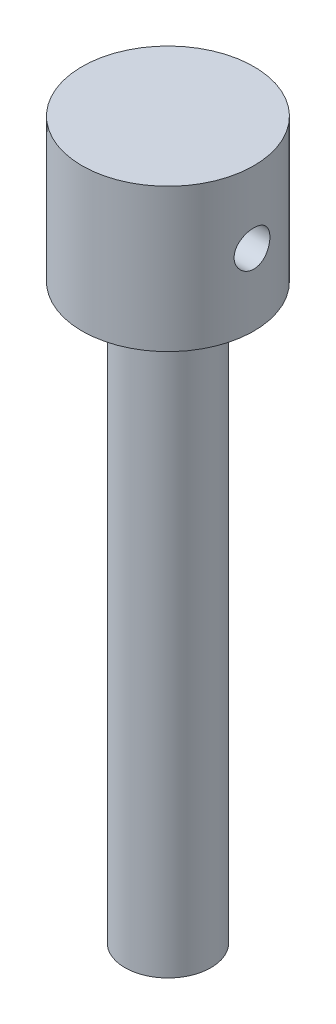
SolidWorks part; units mm, degrees
material "Plain Carbon Steel"
ref_plane "Front Plane" through (0, 0, 0) normal (0, 0, 1) x (1, 0, 0)
ref_plane "Top Plane" through (0, 0, 0) normal (0, 1, 0) x (1, 0, 0)
ref_plane "Right Plane" through (0, 0, 0) normal (1, 0, 0) x (0, 0, -1)
sketch "Shaft Profile" plane through (0, 0, 0) normal (0, 1, 0) x (1, 0, 0)
  circle A0 centre (0, 0) radius 6
  dimension "D1" = 12
extrude "Shaft L80" add sketch "Shaft Profile" along normal blind 80
sketch "Head Profile" plane through (0, 80, 0) normal (0, 1, 0) x (1, 0, 0)
  circle A0 centre (0, 0) radius 12
  dimension "D1" = 24
extrude "Head Ø24 x 20" add sketch "Head Profile" along normal blind 20
sketch "Cross Hole Profile" plane through (0, 0, 0) normal (1, 0, 0) x (0, 0, -1)
  circle A0 centre (0, 90) radius 2.5
  dimension "D1" = 5
  dimension "D2" = 90
extrude "Cross Hole" cut sketch "Cross Hole Profile" against normal mid plane 50
